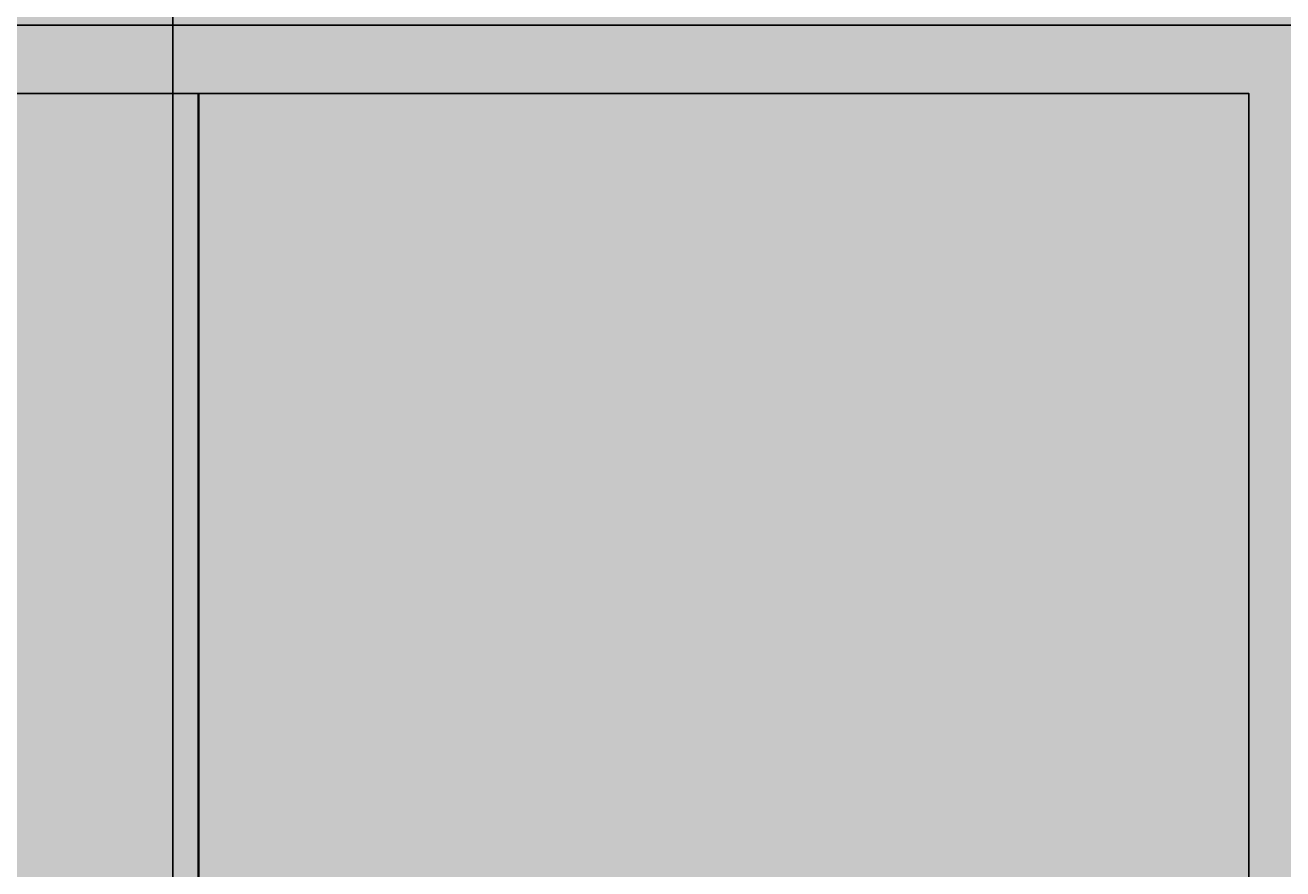
# Model space of a CAD drawing. Units: feet. Extents: x 2695 to 2912, y 795 to 1139.
# Tile 56 of 83: x 2806 to 2843, y 996 to 1021. Entities that reach past the tile are written whole.
import ezdxf

# ---------------------------------------------------------------- set-up
doc = ezdxf.new("R2010")
doc.units = ezdxf.units.FT
for name, color, linetype, lineweight in [('A-ANNO-DIMS', 2, 'Continuous', 18), ('A-ELEV-PATT', 252, 'Continuous', 13), ('A-GLAZ', 4, 'Continuous', 25), ('A-GLAZ-PATT', 254, 'Continuous', 13)]:
    doc.layers.add(name, color=color, linetype=linetype, lineweight=lineweight)
doc.styles.get("Standard").update_dxf_attribs({"font": 'arial.ttf'})
doc.dimstyles.get("Standard").update_dxf_attribs({"dimtxt": 0.18, "dimasz": 0.18, "dimexe": 0.18, "dimexo": 0.0625, "dimgap": 0.09, "dimtad": 0, "dimtih": 1, "dimtoh": 1, "dimdec": 1, "dimzin": 0, "dimdsep": 46, "dimlunit": 3, "dimtxsty": 'Standard', "dimcen": 0.09, "dimadec": 0, "dimazin": 0, "dimtfac": 1, "dimtdec": 1, "dimtofl": 0, "dimtmove": 0, "dimatfit": 3, "dimfxl": 1, "dimtolj": 1, "dimtzin": 0, "dimarcsym": 0})

# ---------------------------------------------------------------- blocks, each defined once
blk = doc.blocks.new('*D49')
at = {"layer": 'A-ANNO-DIMS', "color": 0, "lineweight": -2, "transparency": 16777216}
for p, q in [((2772.522, 972.03), (2772.522, 1138.886)), ((2772.702, 1138.706), (2790.888, 1138.706)), ((2809.861, 1138.706), (2791.674, 1138.706)), ((2810.041, 972.03), (2810.041, 1138.886))]:
    blk.add_line(p, q, dxfattribs=at)
at = {"layer": 'A-ANNO-DIMS', "color": 0, "transparency": 16777216}
for points in [[(2772.702, 1138.736), (2772.702, 1138.676), (2772.522, 1138.706)], [(2809.861, 1138.736), (2809.861, 1138.676), (2810.041, 1138.706)]]:
    blk.add_solid(points, dxfattribs=at)
at = {"layer": 'Defpoints', "color": 0, "transparency": 16777216}
for p in [(2810.041, 1138.706), (2772.522, 971.967), (2810.041, 971.967)]:
    blk.add_point(p, dxfattribs=at)
at = {"layer": 'A-ANNO-DIMS', "color": 0, "transparency": 16777216, "insert": (2791.281, 1138.706), "char_height": 0.18, "attachment_point": 5}
blk.add_mtext('\\A1;37.52', dxfattribs=at)
blk = doc.blocks.new('*D50')
at = {"layer": 'A-ANNO-DIMS', "color": 0, "lineweight": -2, "transparency": 16777216}
for p, q in [((2810.041, 972.03), (2810.041, 1138.886)), ((2810.221, 1138.706), (2848.721, 1138.706)), ((2888.008, 1138.706), (2849.508, 1138.706)), ((2888.188, 972.03), (2888.188, 1138.886))]:
    blk.add_line(p, q, dxfattribs=at)
at = {"layer": 'A-ANNO-DIMS', "color": 0, "transparency": 16777216}
for points in [[(2810.221, 1138.736), (2810.221, 1138.676), (2810.041, 1138.706)], [(2888.008, 1138.736), (2888.008, 1138.676), (2888.188, 1138.706)]]:
    blk.add_solid(points, dxfattribs=at)
at = {"layer": 'Defpoints', "color": 0, "transparency": 16777216}
for p in [(2888.188, 1138.706), (2810.041, 971.967), (2888.188, 971.967)]:
    blk.add_point(p, dxfattribs=at)
at = {"layer": 'A-ANNO-DIMS', "color": 0, "transparency": 16777216, "insert": (2849.114, 1138.706), "char_height": 0.18, "attachment_point": 5}
blk.add_mtext('\\A1;78.15', dxfattribs=at)

msp = doc.modelspace()

# ---------------------------------------------------------------- hatches: boundary and pattern name
at = {"layer": 'A-ELEV-PATT'}
h = msp.add_hatch(color=256, dxfattribs=at)
h.set_gradient(color1=(147, 149, 152), color2=(147, 149, 152), tint=1)
h.paths.add_polyline_path([(2770.6361, 1118.4096), (2710.6361, 1118.4096), (2710.6361, 1062.9306), (2770.6361, 1062.9306)])
h.paths.add_polyline_path([(2890.6361, 1103.3378), (2770.6361, 1103.3378), (2770.6361, 1062.9306), (2890.6361, 1062.9306)])
h.paths.add_polyline_path([(2730.7081, 1048.1052), (2755.1125, 1048.1052), (2755.1125, 936.9306), (2770.6361, 936.9306), (2770.6361, 1050.3105), (2715.8852, 1050.3105), (2715.8852, 936.9306), (2730.7081, 936.9306)])
h.paths.add_polyline_path([(2890.6361, 1050.3105), (2770.6361, 1050.3105), (2770.6361, 971.9673), (2778.0341, 971.9673), (2778.0341, 1020.8235), (2843.575, 1020.8235), (2843.575, 971.9673), (2890.6361, 971.9673)])
h.paths.add_polyline_path([(2888.1882, 970.7156), (2843.575, 970.7156), (2843.575, 964.8267), (2888.1882, 964.8267)])
h.paths.add_polyline_path([(2888.1882, 964.1328), (2843.575, 964.1328), (2843.575, 956.614), (2888.1882, 956.614)])
h.paths.add_polyline_path([(2888.1882, 955.9202), (2843.575, 955.9202), (2843.575, 949.2892), (2888.1882, 949.2892)])
h.paths.add_polyline_path([(2888.1882, 948.5954), (2843.575, 948.5954), (2843.575, 941.3507), (2888.1882, 941.3507)])
h.paths.add_polyline_path([(2888.1882, 940.6569), (2843.575, 940.6569), (2843.575, 936.9306), (2888.1882, 936.9306)])
h.paths.add_polyline_path([(2890.6361, 970.7156), (2888.9368, 970.7156), (2888.9368, 964.8267), (2890.6361, 964.8267)])
h.paths.add_polyline_path([(2890.6361, 964.1328), (2888.9368, 964.1328), (2888.9368, 956.614), (2890.6361, 956.614)])
h.paths.add_polyline_path([(2890.6361, 955.9202), (2888.9368, 955.9202), (2888.9368, 949.2892), (2890.6361, 949.2892)])
h.paths.add_polyline_path([(2890.6361, 940.6569), (2888.9368, 940.6569), (2888.9368, 936.9306), (2890.6361, 936.9306)])
h.paths.add_polyline_path([(2890.6361, 948.5954), (2888.9368, 948.5954), (2888.9368, 941.3507), (2890.6361, 941.3507)])
h.paths.add_polyline_path([(2772.5216, 970.7156), (2770.6361, 970.7156), (2770.6361, 964.8267), (2772.5216, 964.8267)])
h.paths.add_polyline_path([(2772.5216, 964.1328), (2770.6361, 964.1328), (2770.6361, 956.614), (2772.5216, 956.614)])
h.paths.add_polyline_path([(2772.5216, 955.9202), (2770.6361, 955.9202), (2770.6361, 949.2892), (2772.5216, 949.2892)])
h.paths.add_polyline_path([(2772.5216, 948.5954), (2770.6361, 948.5954), (2770.6361, 941.3507), (2772.5216, 941.3507)])
h.paths.add_polyline_path([(2772.5216, 940.6569), (2770.6361, 940.6569), (2770.6361, 936.9306), (2772.5216, 936.9306)])
h.paths.add_polyline_path([(2778.0341, 940.6569), (2773.2702, 940.6569), (2773.2702, 936.9306), (2778.0341, 936.9306)])
h.paths.add_polyline_path([(2778.0341, 970.7156), (2773.2702, 970.7156), (2773.2702, 964.8267), (2778.0341, 964.8267)])
h.paths.add_polyline_path([(2778.0341, 964.1328), (2773.2702, 964.1328), (2773.2702, 956.614), (2778.0341, 956.614)])
h.paths.add_polyline_path([(2778.0341, 955.9202), (2773.2702, 955.9202), (2773.2702, 949.2892), (2778.0341, 949.2892)])
h.paths.add_polyline_path([(2778.0341, 948.5954), (2773.2702, 948.5954), (2773.2702, 941.3507), (2778.0341, 941.3507)])
h.paths.add_polyline_path([(2810.0407, 940.6569), (2780.0341, 940.6569), (2780.0341, 936.9306), (2810.0407, 936.9306)])
h.paths.add_polyline_path([(2890.6361, 924.3105), (2770.6361, 924.3105), (2770.6361, 810.9306), (2773.5029, 810.9306), (2773.5029, 905.5143), (2805.9398, 905.5143), (2838.3767, 905.5143), (2838.3767, 810.9306), (2890.6361, 810.9306)])
h = msp.add_hatch(color=256, dxfattribs=at)
h.set_gradient(color2=(0, 0, 0), tint=1)
h.paths.add_polyline_path([(2772.5216, 971.9673), (2770.6361, 971.9673), (2770.6361, 970.7156), (2772.5216, 970.7156)])
h.paths.add_polyline_path([(2773.2702, 971.9673), (2772.5216, 971.9673), (2772.5216, 970.7156), (2773.2702, 970.7156)])
h.paths.add_polyline_path([(2778.0341, 971.9673), (2773.2702, 971.9673), (2773.2702, 970.7156), (2778.0341, 970.7156)])
h.paths.add_polyline_path([(2780.0341, 971.9673), (2778.0341, 971.9673), (2778.0341, 970.7156), (2780.0341, 970.7156)])
h.paths.add_polyline_path([(2841.575, 971.9673), (2780.0341, 971.9673), (2780.0341, 970.7156), (2841.575, 970.7156)])
h.paths.add_polyline_path([(2843.575, 971.9673), (2841.575, 971.9673), (2841.575, 970.7156), (2843.575, 970.7156)])
h.paths.add_polyline_path([(2888.1882, 971.9673), (2843.575, 971.9673), (2843.575, 970.7156), (2888.1882, 970.7156)])
h.paths.add_polyline_path([(2888.9368, 971.9673), (2888.1882, 971.9673), (2888.1882, 970.7156), (2888.9368, 970.7156)], flags=17)
h.paths.add_polyline_path([(2890.6361, 971.9673), (2888.9368, 971.9673), (2888.9368, 970.7156), (2890.6361, 970.7156)])
h.paths.add_polyline_path([(2888.9368, 971.9673), (2888.1882, 971.9673), (2888.1882, 964.8267), (2888.9368, 964.8267)])
h.paths.add_polyline_path([(2888.9368, 964.8267), (2888.1882, 964.8267), (2888.1882, 964.1328), (2888.9368, 964.1328)])
h.paths.add_polyline_path([(2890.6361, 964.8267), (2888.9368, 964.8267), (2888.9368, 964.1328), (2890.6361, 964.1328)])
h.paths.add_polyline_path([(2888.1882, 964.8267), (2770.6361, 964.8267), (2770.6361, 964.1328), (2888.1882, 964.1328)])
h.paths.add_polyline_path([(2888.9368, 964.1328), (2888.1882, 964.1328), (2888.1882, 936.9306), (2888.9368, 936.9306)])
h.paths.add_polyline_path([(2890.6361, 956.614), (2888.9368, 956.614), (2888.9368, 955.9202), (2890.6361, 955.9202)])
h.paths.add_polyline_path([(2888.1882, 956.614), (2770.6361, 956.614), (2770.6361, 955.9202), (2888.1882, 955.9202)])
h.paths.add_polyline_path([(2890.6361, 949.2892), (2888.9368, 949.2892), (2888.9368, 948.5954), (2890.6361, 948.5954)])
h.paths.add_polyline_path([(2888.1882, 949.2892), (2770.6361, 949.2892), (2770.6361, 948.5954), (2888.1882, 948.5954)])
h.paths.add_polyline_path([(2890.6361, 941.3507), (2888.9368, 941.3507), (2888.9368, 940.6569), (2890.6361, 940.6569)])
h.paths.add_polyline_path([(2888.1882, 941.3507), (2770.6361, 941.3507), (2770.6361, 940.6569), (2888.1882, 940.6569)])
h.paths.add_polyline_path([(2773.2702, 970.7156), (2772.5216, 970.7156), (2772.5216, 964.8267), (2773.2702, 964.8267)])
h.paths.add_polyline_path([(2773.2702, 964.1328), (2772.5216, 964.1328), (2772.5216, 956.614), (2773.2702, 956.614)])
h.paths.add_polyline_path([(2773.2702, 955.9202), (2772.5216, 955.9202), (2772.5216, 936.9306), (2773.2702, 936.9306)])
h.paths.add_polyline_path([(2810.7893, 970.7156), (2810.0407, 970.7156), (2810.0407, 964.8267), (2810.7893, 964.8267)], flags=17)
h.paths.add_polyline_path([(2810.7893, 964.1328), (2810.0407, 964.1328), (2810.0407, 956.614), (2810.7893, 956.614)], flags=17)
h.paths.add_polyline_path([(2810.7893, 955.9202), (2810.0407, 955.9202), (2810.0407, 949.2892), (2810.7893, 949.2892)], flags=17)
h.paths.add_polyline_path([(2810.7893, 971.9673), (2810.0407, 971.9673), (2810.0407, 941.3507), (2810.7893, 941.3507)])
h.paths.add_polyline_path([(2810.7893, 940.6569), (2810.0407, 940.6569), (2810.0407, 936.9306), (2810.7893, 936.9306)])
h.paths.add_polyline_path([(2780.0341, 1018.8235), (2841.575, 1018.8235), (2841.575, 971.9673), (2843.575, 971.9673), (2843.575, 1020.8235), (2778.0341, 1020.8235), (2778.0341, 971.9673), (2780.0341, 971.9673)])
h.paths.add_polyline_path([(2780.0341, 970.7156), (2778.0341, 970.7156), (2778.0341, 964.8267), (2780.0341, 964.8267)])
h.paths.add_polyline_path([(2780.0341, 964.1328), (2778.0341, 964.1328), (2778.0341, 956.614), (2780.0341, 956.614)])
h.paths.add_polyline_path([(2780.0341, 955.9202), (2778.0341, 955.9202), (2778.0341, 949.2892), (2780.0341, 949.2892)])
h.paths.add_polyline_path([(2780.0341, 948.5954), (2778.0341, 948.5954), (2778.0341, 941.3507), (2780.0341, 941.3507)])
h.paths.add_polyline_path([(2780.0341, 940.6569), (2778.0341, 940.6569), (2778.0341, 936.9306), (2780.0341, 936.9306)])
h.paths.add_polyline_path([(2843.575, 940.6569), (2841.575, 940.6569), (2841.575, 936.9306), (2843.575, 936.9306)])
h.paths.add_polyline_path([(2843.575, 948.5954), (2841.575, 948.5954), (2841.575, 941.3507), (2843.575, 941.3507)])
h.paths.add_polyline_path([(2843.575, 970.7156), (2841.575, 970.7156), (2841.575, 964.8267), (2843.575, 964.8267)])
h.paths.add_polyline_path([(2843.575, 964.1328), (2841.575, 964.1328), (2841.575, 956.614), (2843.575, 956.614)])
h.paths.add_polyline_path([(2843.575, 955.9202), (2841.575, 955.9202), (2841.575, 949.2892), (2843.575, 949.2892)])
h.paths.add_polyline_path([(2805.0538, 874.1057), (2803.9681, 874.1057), (2803.9681, 846.2857), (2805.0538, 846.2857)])
h.paths.add_polyline_path([(2758.1515, 902.577), (2724.1893, 902.577), (2724.1893, 874.8571), (2758.1515, 874.8571)])
h.paths.add_polyline_path([(2726.1893, 900.577), (2756.1515, 900.577), (2756.1515, 876.8571), (2726.1893, 876.8571)], flags=16)
h.paths.add_polyline_path([(2740.7302, 900.577), (2741.6105, 900.577), (2741.6105, 876.8571), (2740.7302, 876.8571)], flags=0)
at = {"layer": 'A-GLAZ-PATT'}
h = msp.add_hatch(color=256, dxfattribs=at)
h.set_gradient(color1=(213, 227, 240), color2=(213, 227, 240))
h.paths.add_polyline_path([(2810.8045, 1018.8235), (2780.0341, 1018.8235), (2780.0341, 971.9673), (2810.8045, 971.9673)])
h.paths.add_polyline_path([(2841.575, 1018.8235), (2810.8045, 1018.8235), (2810.8045, 971.9673), (2841.575, 971.9673)])
h.paths.add_polyline_path([(2810.0407, 970.7156), (2780.0341, 970.7156), (2780.0341, 964.8267), (2810.0407, 964.8267)])
h.paths.add_polyline_path([(2841.575, 970.7156), (2810.8045, 970.7156), (2810.8045, 964.8267), (2841.575, 964.8267)])
h.paths.add_polyline_path([(2841.575, 964.1328), (2810.8045, 964.1328), (2810.8045, 956.614), (2841.575, 956.614)])
h.paths.add_polyline_path([(2810.0407, 964.1328), (2780.0341, 964.1328), (2780.0341, 956.614), (2810.0407, 956.614)])
h.paths.add_polyline_path([(2810.0407, 955.9202), (2780.0341, 955.9202), (2780.0341, 949.2892), (2810.0407, 949.2892)])
h.paths.add_polyline_path([(2841.575, 955.9202), (2810.8045, 955.9202), (2810.8045, 949.2892), (2841.575, 949.2892)])
h.paths.add_polyline_path([(2841.575, 948.5954), (2810.8045, 948.5954), (2810.8045, 941.3507), (2841.575, 941.3507)])
h.paths.add_polyline_path([(2810.0407, 948.5954), (2780.0341, 948.5954), (2780.0341, 941.3507), (2810.0407, 941.3507)])
h.paths.add_polyline_path([(2810.0407, 940.6569), (2780.0341, 940.6569), (2780.0341, 936.9306), (2810.0407, 936.9306)])
h.paths.add_polyline_path([(2841.575, 940.6569), (2810.8045, 940.6569), (2810.8045, 936.9306), (2841.575, 936.9306)])

# ---------------------------------------------------------------- linework, layer by layer
at = {"layer": 'A-GLAZ'}
msp.add_line((2810.8045, 1018.8235), (2810.8045, 971.9673), dxfattribs=at)
for points in [[(2778.0341, 936.9306), (2778.0341, 1020.8235), (2843.575, 1020.8235), (2843.575, 936.9306)], [(2780.0341, 936.9306), (2780.0341, 1018.8235), (2841.575, 1018.8235), (2841.575, 936.9306)]]:
    msp.add_lwpolyline(points, dxfattribs=at)
for points in [[(2810.8045, 1018.8235), (2810.7893, 1018.8235), (2810.7893, 971.9673), (2810.8045, 971.9673)], [(2810.8045, 1018.8235), (2810.7893, 1018.8235), (2810.7893, 936.9306), (2810.8045, 936.9306)], [(2810.8045, 1018.8235), (2810.8045, 1018.8235), (2810.8045, 936.9306), (2810.8045, 936.9306)]]:
    msp.add_lwpolyline(points, close=True, dxfattribs=at)

# ---------------------------------------------------------------- dimensions: what is measured, and where the dimension line sits
at = {"layer": 'A-ANNO-DIMS'}
for base, p1, p2, picture, middle in [((2810.0407, 1138.7056), (2772.5216, 971.9673), (2810.0407, 971.9673), '*D49', (2791.2811, 1138.7056)), ((2888.1882, 1138.7056), (2810.0407, 971.9673), (2888.1882, 971.9673), '*D50', (2849.1144, 1138.7056))]:
    dim = msp.add_linear_dim(base=base, p1=p1, p2=p2, dimstyle='Standard', override={"dimdec": 2, "dimlfac": 1, "dimrnd": 0, "dimzin": 0, "dimdsep": 46, "dimlunit": 2}, dxfattribs=at)
    dim.commit()
    dim.dimension.update_dxf_attribs({"geometry": picture, "text_midpoint": middle})

doc.saveas('drawing.dxf')
